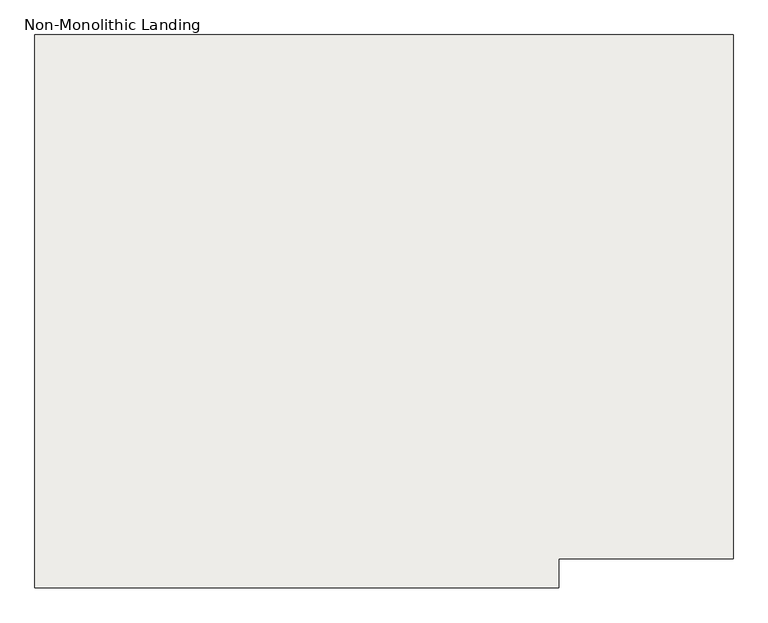
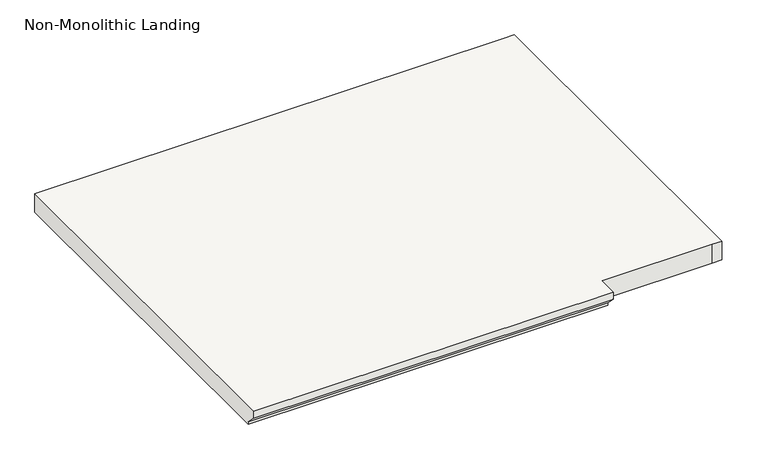
"""IFC4 building model written with IfcOpenShell, lengths in millimetres: slab geometry, Non-Monolithic Landing."""

from ifc_helpers import new_model, si_unit, origin, place, context, project, spatial, faceted_brep, source, transform, mapped, element, save


def non_monolithic_landing_db9d561b(model_context):
    return source(origin(), model_context, "Body", "Brep", [
        faceted_brep([(-12594.3954771, 2713.6129676, 4425.95), (-12594.3954771, 2713.6129676, 4445.0), (-13508.7954771, 2713.6129676, 4445.0), (-13508.7954771, 2713.6129676, 4425.95), (-12594.3954771, 2739.0129676, 4400.55), (-13508.7954771, 2739.0129676, 4400.55), (-12594.3954771, 2764.4129676, 4445.0), (-12314.9954771, 2764.4129676, 4445.0), (-12289.5954771, 2764.4129676, 4445.0), (-12289.5954771, 3678.8129676, 4445.0), (-12314.9954771, 3678.8129676, 4445.0), (-13508.7954771, 3678.8129676, 4445.0), (-12594.3954771, 2739.0129676, 4394.2), (-13508.7954771, 2739.0129676, 4394.2), (-13508.7954771, 3678.8129676, 4394.2), (-12314.9954771, 3678.8129676, 4394.2), (-12289.5954771, 3678.8129676, 4394.2), (-12289.5954771, 2764.4129676, 4394.2), (-12314.9954771, 2764.4129676, 4394.2), (-12594.3954771, 2764.4129676, 4394.2)], [[[0, 1, 2, 3]], [[4, 0, 3, 5]], [[6, 7, 8, 9, 10, 11, 2, 1]], [[12, 13, 14, 15, 16, 17, 18, 19]], [[13, 12, 4, 5]], [[6, 1, 0, 4, 12, 19]], [[7, 6, 19, 18]], [[8, 7, 18, 17]], [[9, 8, 17, 16]], [[10, 9, 16, 15]], [[11, 10, 15, 14]], [[2, 11, 14, 13, 5, 3]]]),
    ])


if __name__ == "__main__":
    model = new_model("IFC4")
    model_context = context("Model", 3, world=origin())
    ifc_project = project(units=[si_unit("LENGTHUNIT", "METRE", prefix="MILLI")], contexts=[model_context])
    site = spatial("IfcSite", under=ifc_project)
    building = spatial("IfcBuilding", under=site)
    placement = place(None, origin())
    non_monolithic_landing_shape = non_monolithic_landing_db9d561b(model_context)
    element("IfcSlab", 1, ObjectType="Non-Monolithic Landing", at=placement, inside=building, context=model_context, shape_type="MappedRepresentation", body=[
        mapped(non_monolithic_landing_shape, transform((0.0, 0.0, 0.0), x_axis=(1.0, 0.0, 0.0), y_axis=(0.0, 1.0, 0.0), z_axis=(0.0, 0.0, 1.0))),
    ])
    save(model, "model.ifc")
